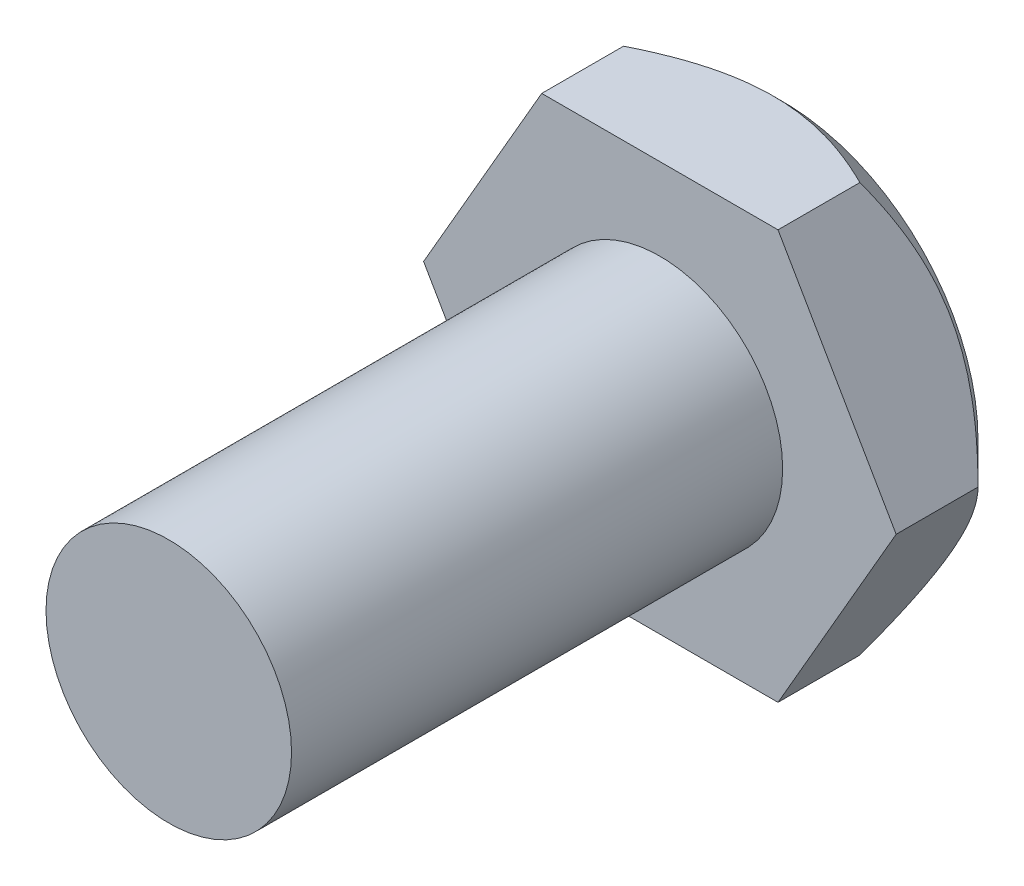
SolidWorks part; units mm, degrees
material "Plain Carbon Steel"
ref_plane "Front Plane" through (0, 0, 0) normal (0, 0, 1) x (1, 0, 0)
ref_plane "Top Plane" through (0, 0, 0) normal (0, 1, 0) x (1, 0, 0)
ref_plane "Right Plane" through (0, 0, 0) normal (1, 0, 0) x (0, 0, -1)
sketch "Hex Head Profile 10AF" plane through (0, 0, 0) normal (0, 0, 1) x (1, 0, 0)
  line L1 (-2.8868, 5) -> (-5.7735, 0)
  line L2 (-5.7735, 0) -> (-2.8868, -5)
  line L3 (-2.8868, -5) -> (2.8868, -5)
  line L4 (2.8868, -5) -> (5.7735, 0)
  line L5 (5.7735, 0) -> (2.8868, 5)
  line L6 (2.8868, 5) -> (-2.8868, 5)
  circle A0 centre (0, 0) radius 5 construction
  dimension "D1" = 10
extrude "Hex Head" add sketch "Hex Head Profile 10AF" along normal blind 3
sketch "Shank Profile Ø6" plane through (0, 0, 3) normal (0, 0, 1) x (1, 0, 0)
  circle A0 centre (0, 0) radius 3
  dimension "D1" = 6
extrude "Shank Ø6x12" add sketch "Shank Profile Ø6" along normal blind 12
cosmetic thread "Cosmetic Thread1" parameters "D2"=4.891
cosmetic thread "Cosmetic Thread2" parameters "D2"=4.891
sketch "Head Chamfer Profile" plane through (0, 0, 0) normal (0, 1, 0) x (1, 0, 0)
  line L0 (0, 2.7759) -> (0, -4.5237) construction
  line L1 (-4.7735, 0) -> (-5.7735, 0)
  line L2 (-2.8868, 0) -> (-5.7735, 0) construction
  line L3 (-5.7735, 0) -> (-5.7735, -1)
  line L4 (-5.7735, -3) -> (-5.7735, 0) construction
  line L5 (-5.7735, -1) -> (-4.7735, 0)
  dimension "D1" = 45
  dimension "D2" = 1
revolve "Head Chamfer 45x1" cut sketch "Head Chamfer Profile" angle 360 about L0
